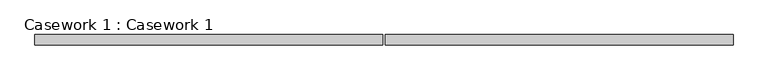
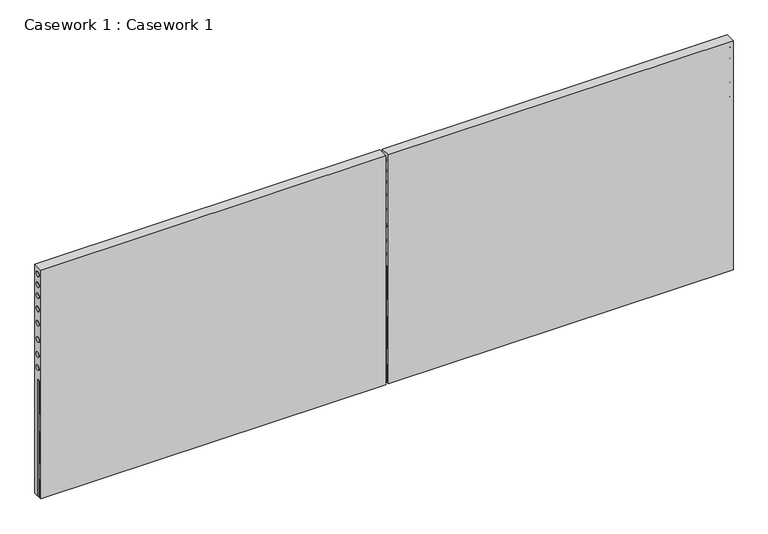
"""IFC4 building model written with IfcOpenShell, lengths in millimetres: furniture geometry, Casework 1 : Casework 1."""

from ifc_helpers import new_model, si_unit, point, frame, frame_2d, origin, place, context, project, spatial, polyline, circle_curve, trimmed, segment, composite_curve, outline, extrude, source, transform, mapped, element, save


def casework_1_casework_1_032930e3(model_context):
    return source(origin(), model_context, "Body", "SweptSolid", [
        extrude(outline(polyline([(-7871.0142637, 627.9554688), (-7871.0142637, 12.0054688), (-7877.3642637, 12.0054688), (-7883.7142637, 12.0054688), (-7883.7142637, 107.2554688), (-7877.3642637, 107.2554688), (-7877.3642637, 189.8054688), (-7883.7142637, 189.8054688), (-7883.7142637, 361.2554688), (-7877.3642637, 361.2554688), (-7877.3642637, 450.1554688), (-7883.7142637, 450.1554688), (-7883.7142637, 627.9554688), (-7871.0142637, 627.9554688)])), frame((-6509.964062, 0.0, 0.0), z_axis=(1.0, 0.0, 0.0), x_axis=(0.0, 1.0, 0.0)), (0.0, 0.0, 1.0), 1720.85),
        extrude(outline(composite_curve([segment(trimmed(circle_curve(frame_2d((-7868.8975515, 1181.8055707)), 12.7), [point((-7868.8975515, 1194.5055707))], [point((-7868.8975515, 1169.1055707))], False, "CARTESIAN"), True, "CONTINUOUS"), segment(trimmed(circle_curve(frame_2d((-7868.8975515, 1181.8055707)), 12.7), [point((-7868.8975515, 1169.1055707))], [point((-7868.8975515, 1194.5055707))], False, "CARTESIAN"), True, "CONTINUOUS")], self_intersect=False)), frame((-6509.964062, 0.0, 0.0), z_axis=(1.0, 0.0, 0.0), x_axis=(0.0, 1.0, 0.0)), (0.0, 0.0, 1.0), 1720.85),
        extrude(outline(composite_curve([segment(trimmed(circle_curve(frame_2d((-7868.8975515, 1124.6555707)), 12.7), [point((-7868.8975515, 1137.3555707))], [point((-7868.8975515, 1111.9555707))], False, "CARTESIAN"), True, "CONTINUOUS"), segment(trimmed(circle_curve(frame_2d((-7868.8975515, 1124.6555707)), 12.7), [point((-7868.8975515, 1111.9555707))], [point((-7868.8975515, 1137.3555707))], False, "CARTESIAN"), True, "CONTINUOUS")], self_intersect=False)), frame((-6509.964062, 0.0, 0.0), z_axis=(1.0, 0.0, 0.0), x_axis=(0.0, 1.0, 0.0)), (0.0, 0.0, 1.0), 1720.85),
        extrude(outline(composite_curve([segment(trimmed(circle_curve(frame_2d((-7868.8975515, 1067.5055707)), 12.7), [point((-7868.8975515, 1080.2055707))], [point((-7868.8975515, 1054.8055707))], False, "CARTESIAN"), True, "CONTINUOUS"), segment(trimmed(circle_curve(frame_2d((-7868.8975515, 1067.5055707)), 12.7), [point((-7868.8975515, 1054.8055707))], [point((-7868.8975515, 1080.2055707))], False, "CARTESIAN"), True, "CONTINUOUS")], self_intersect=False)), frame((-6509.964062, 0.0, 0.0), z_axis=(1.0, 0.0, 0.0), x_axis=(0.0, 1.0, 0.0)), (0.0, 0.0, 1.0), 1720.85),
        extrude(outline(composite_curve([segment(trimmed(circle_curve(frame_2d((-7868.8975515, 997.6555707)), 12.7), [point((-7868.8975515, 1010.3555707))], [point((-7868.8975515, 984.9555707))], False, "CARTESIAN"), True, "CONTINUOUS"), segment(trimmed(circle_curve(frame_2d((-7868.8975515, 997.6555707)), 12.7), [point((-7868.8975515, 984.9555707))], [point((-7868.8975515, 1010.3555707))], False, "CARTESIAN"), True, "CONTINUOUS")], self_intersect=False)), frame((-6509.964062, 0.0, 0.0), z_axis=(1.0, 0.0, 0.0), x_axis=(0.0, 1.0, 0.0)), (0.0, 0.0, 1.0), 1720.85),
        extrude(outline(composite_curve([segment(trimmed(circle_curve(frame_2d((-7868.8975515, 921.4555707)), 12.7), [point((-7868.8975515, 934.1555707))], [point((-7868.8975515, 908.7555707))], False, "CARTESIAN"), True, "CONTINUOUS"), segment(trimmed(circle_curve(frame_2d((-7868.8975515, 921.4555707)), 12.7), [point((-7868.8975515, 908.7555707))], [point((-7868.8975515, 934.1555707))], False, "CARTESIAN"), True, "CONTINUOUS")], self_intersect=False)), frame((-6509.964062, 0.0, 0.0), z_axis=(1.0, 0.0, 0.0), x_axis=(0.0, 1.0, 0.0)), (0.0, 0.0, 1.0), 1720.85),
        extrude(outline(composite_curve([segment(trimmed(circle_curve(frame_2d((-7870.223752, 836.547442)), 12.7), [point((-7870.223752, 849.247442))], [point((-7870.223752, 823.847442))], False, "CARTESIAN"), True, "CONTINUOUS"), segment(trimmed(circle_curve(frame_2d((-7870.223752, 836.547442)), 12.7), [point((-7870.223752, 823.847442))], [point((-7870.223752, 849.247442))], False, "CARTESIAN"), True, "CONTINUOUS")], self_intersect=False)), frame((-6509.964062, 0.0, 0.0), z_axis=(1.0, 0.0, 0.0), x_axis=(0.0, 1.0, 0.0)), (0.0, 0.0, 1.0), 1720.85),
        extrude(outline(composite_curve([segment(trimmed(circle_curve(frame_2d((-7868.4584753, 756.3711513)), 12.7), [point((-7868.4584753, 769.0711513))], [point((-7868.4584753, 743.6711513))], False, "CARTESIAN"), True, "CONTINUOUS"), segment(trimmed(circle_curve(frame_2d((-7868.4584753, 756.3711513)), 12.7), [point((-7868.4584753, 743.6711513))], [point((-7868.4584753, 769.0711513))], False, "CARTESIAN"), True, "CONTINUOUS")], self_intersect=False)), frame((-6509.964062, 0.0, 0.0), z_axis=(1.0, 0.0, 0.0), x_axis=(0.0, 1.0, 0.0)), (0.0, 0.0, 1.0), 1720.85),
        extrude(outline(composite_curve([segment(trimmed(circle_curve(frame_2d((-7868.4031216, 687.1148071)), 12.7), [point((-7868.4031216, 699.8148071))], [point((-7868.4031216, 674.4148071))], False, "CARTESIAN"), True, "CONTINUOUS"), segment(trimmed(circle_curve(frame_2d((-7868.4031216, 687.1148071)), 12.7), [point((-7868.4031216, 674.4148071))], [point((-7868.4031216, 699.8148071))], False, "CARTESIAN"), True, "CONTINUOUS")], self_intersect=False)), frame((-6509.964062, 0.0, 0.0), z_axis=(1.0, 0.0, 0.0), x_axis=(0.0, 1.0, 0.0)), (0.0, 0.0, 1.0), 1720.85),
        extrude(outline(polyline([(-7871.0142637, 627.9554688), (-7871.0142637, 12.0054688), (-7877.3642637, 12.0054688), (-7883.7142637, 12.0054688), (-7883.7142637, 107.2554687), (-7877.3642637, 107.2554687), (-7877.3642637, 189.8054687), (-7883.7142637, 189.8054687), (-7883.7142637, 361.2554687), (-7877.3642637, 361.2554687), (-7877.3642637, 450.1554687), (-7883.7142637, 450.1554687), (-7883.7142637, 627.9554688), (-7871.0142637, 627.9554688)])), frame((-4776.414062, 0.0, 0.0), z_axis=(1.0, 0.0, 0.0), x_axis=(0.0, 1.0, 0.0)), (0.0, 0.0, 1.0), 1720.85),
        extrude(outline(composite_curve([segment(trimmed(circle_curve(frame_2d((-7868.8975515, 1181.8055707)), 12.7), [point((-7868.8975515, 1194.5055707))], [point((-7868.8975515, 1169.1055707))], False, "CARTESIAN"), True, "CONTINUOUS"), segment(trimmed(circle_curve(frame_2d((-7868.8975515, 1181.8055707)), 12.7), [point((-7868.8975515, 1169.1055707))], [point((-7868.8975515, 1194.5055707))], False, "CARTESIAN"), True, "CONTINUOUS")], self_intersect=False)), frame((-4776.414062, 0.0, 0.0), z_axis=(1.0, 0.0, 0.0), x_axis=(0.0, 1.0, 0.0)), (0.0, 0.0, 1.0), 1720.85),
        extrude(outline(composite_curve([segment(trimmed(circle_curve(frame_2d((-7868.8975515, 1124.6555707)), 12.7), [point((-7868.8975515, 1137.3555707))], [point((-7868.8975515, 1111.9555707))], False, "CARTESIAN"), True, "CONTINUOUS"), segment(trimmed(circle_curve(frame_2d((-7868.8975515, 1124.6555707)), 12.7), [point((-7868.8975515, 1111.9555707))], [point((-7868.8975515, 1137.3555707))], False, "CARTESIAN"), True, "CONTINUOUS")], self_intersect=False)), frame((-4776.414062, 0.0, 0.0), z_axis=(1.0, 0.0, 0.0), x_axis=(0.0, 1.0, 0.0)), (0.0, 0.0, 1.0), 1720.85),
        extrude(outline(composite_curve([segment(trimmed(circle_curve(frame_2d((-7868.8975515, 1067.5055707)), 12.7), [point((-7868.8975515, 1080.2055707))], [point((-7868.8975515, 1054.8055707))], False, "CARTESIAN"), True, "CONTINUOUS"), segment(trimmed(circle_curve(frame_2d((-7868.8975515, 1067.5055707)), 12.7), [point((-7868.8975515, 1054.8055707))], [point((-7868.8975515, 1080.2055707))], False, "CARTESIAN"), True, "CONTINUOUS")], self_intersect=False)), frame((-4776.414062, 0.0, 0.0), z_axis=(1.0, 0.0, 0.0), x_axis=(0.0, 1.0, 0.0)), (0.0, 0.0, 1.0), 1720.85),
        extrude(outline(composite_curve([segment(trimmed(circle_curve(frame_2d((-7868.8975515, 997.6555707)), 12.7), [point((-7868.8975515, 1010.3555707))], [point((-7868.8975515, 984.9555707))], False, "CARTESIAN"), True, "CONTINUOUS"), segment(trimmed(circle_curve(frame_2d((-7868.8975515, 997.6555707)), 12.7), [point((-7868.8975515, 984.9555707))], [point((-7868.8975515, 1010.3555707))], False, "CARTESIAN"), True, "CONTINUOUS")], self_intersect=False)), frame((-4776.414062, 0.0, 0.0), z_axis=(1.0, 0.0, 0.0), x_axis=(0.0, 1.0, 0.0)), (0.0, 0.0, 1.0), 1720.85),
        extrude(outline(composite_curve([segment(trimmed(circle_curve(frame_2d((-7868.8975515, 921.4555707)), 12.7), [point((-7868.8975515, 934.1555707))], [point((-7868.8975515, 908.7555707))], False, "CARTESIAN"), True, "CONTINUOUS"), segment(trimmed(circle_curve(frame_2d((-7868.8975515, 921.4555707)), 12.7), [point((-7868.8975515, 908.7555707))], [point((-7868.8975515, 934.1555707))], False, "CARTESIAN"), True, "CONTINUOUS")], self_intersect=False)), frame((-4776.414062, 0.0, 0.0), z_axis=(1.0, 0.0, 0.0), x_axis=(0.0, 1.0, 0.0)), (0.0, 0.0, 1.0), 1720.85),
        extrude(outline(composite_curve([segment(trimmed(circle_curve(frame_2d((-7870.223752, 836.547442)), 12.7), [point((-7870.223752, 849.247442))], [point((-7870.223752, 823.847442))], False, "CARTESIAN"), True, "CONTINUOUS"), segment(trimmed(circle_curve(frame_2d((-7870.223752, 836.547442)), 12.7), [point((-7870.223752, 823.847442))], [point((-7870.223752, 849.247442))], False, "CARTESIAN"), True, "CONTINUOUS")], self_intersect=False)), frame((-4776.414062, 0.0, 0.0), z_axis=(1.0, 0.0, 0.0), x_axis=(0.0, 1.0, 0.0)), (0.0, 0.0, 1.0), 1720.85),
        extrude(outline(composite_curve([segment(trimmed(circle_curve(frame_2d((-7868.4584753, 756.3711513)), 12.7), [point((-7868.4584753, 769.0711513))], [point((-7868.4584753, 743.6711513))], False, "CARTESIAN"), True, "CONTINUOUS"), segment(trimmed(circle_curve(frame_2d((-7868.4584753, 756.3711513)), 12.7), [point((-7868.4584753, 743.6711513))], [point((-7868.4584753, 769.0711513))], False, "CARTESIAN"), True, "CONTINUOUS")], self_intersect=False)), frame((-4776.414062, 0.0, 0.0), z_axis=(1.0, 0.0, 0.0), x_axis=(0.0, 1.0, 0.0)), (0.0, 0.0, 1.0), 1720.85),
        extrude(outline(composite_curve([segment(trimmed(circle_curve(frame_2d((-7868.4031216, 687.1148071)), 12.7), [point((-7868.4031216, 699.8148071))], [point((-7868.4031216, 674.4148071))], False, "CARTESIAN"), True, "CONTINUOUS"), segment(trimmed(circle_curve(frame_2d((-7868.4031216, 687.1148071)), 12.7), [point((-7868.4031216, 674.4148071))], [point((-7868.4031216, 699.8148071))], False, "CARTESIAN"), True, "CONTINUOUS")], self_intersect=False)), frame((-4776.414062, 0.0, 0.0), z_axis=(1.0, 0.0, 0.0), x_axis=(0.0, 1.0, 0.0)), (0.0, 0.0, 1.0), 1720.85),
        extrude(outline(polyline([(-4789.114062, -7896.4142637), (-6509.964062, -7896.4142637), (-6509.964062, -7845.6142637), (-4789.114062, -7845.6142637), (-4789.114062, -7896.4142637)])), frame((0.0, 0.0, 12.0054688), z_axis=(0.0, 0.0, 1.0), x_axis=(1.0, 0.0, 0.0)), (0.0, 0.0, 1.0), 1207.1945312),
        extrude(outline(polyline([(-3055.564062, -7896.4142637), (-4776.414062, -7896.4142637), (-4776.414062, -7845.6142637), (-3055.564062, -7845.6142637), (-3055.564062, -7896.4142637)])), frame((0.0, 0.0, 12.0054688), z_axis=(0.0, 0.0, 1.0), x_axis=(1.0, 0.0, 0.0)), (0.0, 0.0, 1.0), 1207.1945312),
    ])


if __name__ == "__main__":
    model = new_model("IFC4")
    model_context = context("Model", 3, world=origin())
    ifc_project = project(units=[si_unit("LENGTHUNIT", "METRE", prefix="MILLI")], contexts=[model_context])
    site = spatial("IfcSite", under=ifc_project)
    building = spatial("IfcBuilding", under=site)
    placement = place(None, origin())
    casework_1_casework_1_shape = casework_1_casework_1_032930e3(model_context)
    element("IfcFurniture", 1, ObjectType="Casework 1 : Casework 1", at=placement, inside=building, context=model_context, shape_type="MappedRepresentation", body=[
        mapped(casework_1_casework_1_shape, transform((0.0, 0.0, 0.0), x_axis=(1.0, 0.0, 0.0), y_axis=(0.0, 1.0, 0.0), z_axis=(0.0, 0.0, 1.0))),
    ])
    save(model, "model.ifc")

# Revit data of these elements
# Element 1 (IfcFurniture, "Casework 1 : Casework 1")
#   Materials on its faces: "Iron, Ductile", "Door - Frame"
# Materials
#   "Iron, Ductile": class "Metal", colour RGB 0 0 0, transparency 0, Description = "Ductile cast iron", Cost = 0
#   "Door - Frame": colour RGB 118 70 51, transparency 0, Cost = 0
